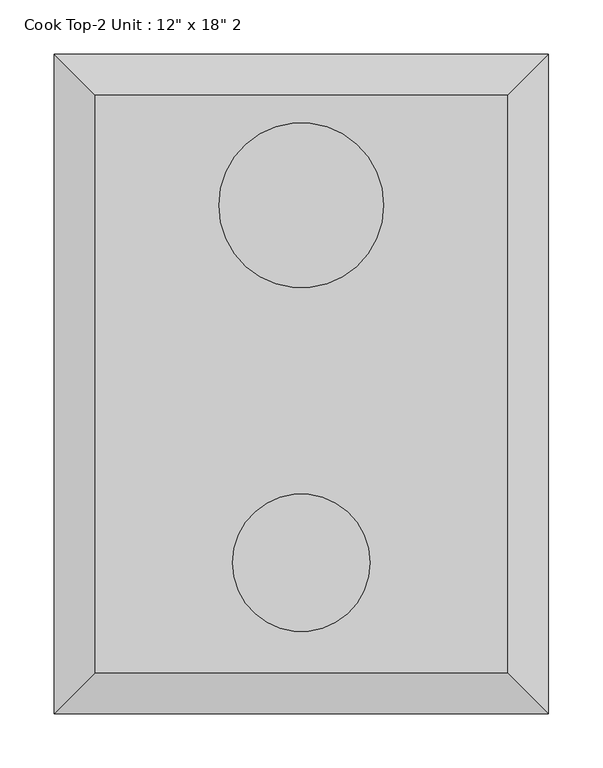
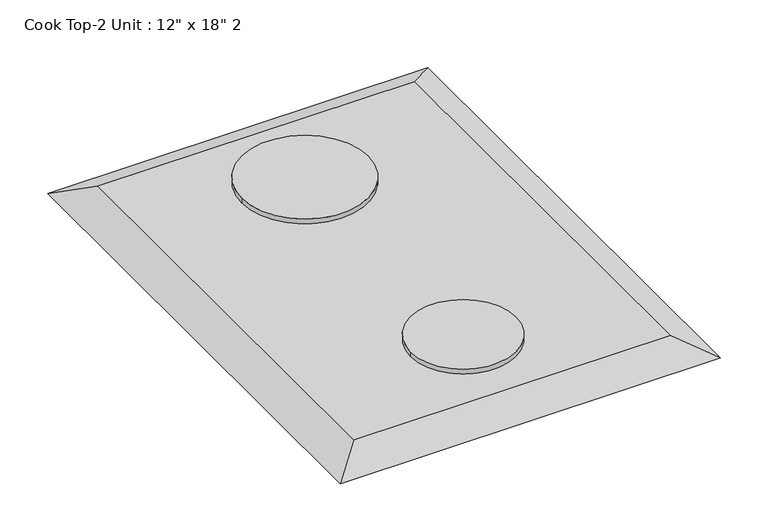
"""IFC4 building model written with IfcOpenShell, lengths in millimetres: proxy geometry."""

from ifc_helpers import new_model, si_unit, point, frame, frame_2d, origin, place, context, project, spatial, circle_curve, trimmed, segment, composite_curve, outline, extrude, faceted_brep, source, transform, mapped, element, save


def proxy_3c1fa1d0(model_context):
    return source(origin(), model_context, "Body", "SolidModel", [
        faceted_brep([(266.7, 296.9247956, 933.45), (-114.3, 296.9247956, 933.45), (-114.3, -236.4752044, 933.45), (266.7, -236.4752044, 933.45), (304.8, 335.0247956, 914.4), (304.8, -274.5752044, 914.4), (-152.4, -274.5752044, 914.4), (-152.4, 335.0247956, 914.4)], [[[0, 1, 2, 3]], [[4, 5, 6, 7]], [[4, 7, 1, 0]], [[7, 6, 2, 1]], [[6, 5, 3, 2]], [[5, 4, 0, 3]]]),
        extrude(outline(composite_curve([segment(trimmed(circle_curve(frame_2d((76.2, 195.3247956)), 76.2), [point((152.4, 195.3247956))], [point((0.0, 195.3247956))], False, "CARTESIAN"), True, "CONTINUOUS"), segment(trimmed(circle_curve(frame_2d((76.2, 195.3247956)), 76.2), [point((0.0, 195.3247956))], [point((152.4, 195.3247956))], False, "CARTESIAN"), True, "CONTINUOUS")], self_intersect=False)), frame((0.0, 0.0, 933.45), z_axis=(0.0, 0.0, 1.0), x_axis=(1.0, 0.0, 0.0)), (0.0, 0.0, 1.0), 6.35),
        extrude(outline(composite_curve([segment(trimmed(circle_curve(frame_2d((76.2, -134.8752044)), 63.5), [point((139.7, -134.8752044))], [point((12.7, -134.8752044))], False, "CARTESIAN"), True, "CONTINUOUS"), segment(trimmed(circle_curve(frame_2d((76.2, -134.8752044)), 63.5), [point((12.7, -134.8752044))], [point((139.7, -134.8752044))], False, "CARTESIAN"), True, "CONTINUOUS")], self_intersect=False)), frame((0.0, 0.0, 933.45), z_axis=(0.0, 0.0, 1.0), x_axis=(1.0, 0.0, 0.0)), (0.0, 0.0, 1.0), 6.35),
    ])


if __name__ == "__main__":
    model = new_model("IFC4")
    model_context = context("Model", 3, world=origin())
    ifc_project = project(units=[si_unit("LENGTHUNIT", "METRE", prefix="MILLI")], contexts=[model_context])
    site = spatial("IfcSite", under=ifc_project)
    building = spatial("IfcBuilding", under=site)
    placement = place(None, origin())
    proxy_shape = proxy_3c1fa1d0(model_context)
    element("IfcBuildingElementProxy", 1, Name="Cook Top-2 Unit : 12\" x 18\" 2", ObjectType="Cook Top-2 Unit : 12\" x 18\" 2", at=placement, inside=building, context=model_context, shape_type="MappedRepresentation", body=[
        mapped(proxy_shape, transform((0.0, 0.0, 0.0), x_axis=(1.0, 0.0, 0.0), y_axis=(0.0, 1.0, 0.0), z_axis=(0.0, 0.0, 1.0))),
    ])
    save(model, "model.ifc")

# Revit data of these elements
# Type "Cook Top-2 Unit : 12\" x 18\" 2"
#   Assembly Code = "E1090400"
#   Counter Height = 3' - 0"
#   Depth = 2' - 0"
#   Width = 1' - 6"
#   Burner Material = Metal - Chrome
#   Cooktop Material = Metal - Steel, Polished
#   Default Elevation = 0
# Element 1 (IfcBuildingElementProxy, "Cook Top-2 Unit : 12\" x 18\" 2")
#   Materials on its faces: "Metal - Steel, Polished", "Metal - Chrome"
# Materials
#   "Metal - Chrome": colour RGB 57 57 57, transparency 0
#   "Metal - Steel, Polished": colour RGB 57 57 57, transparency 0
